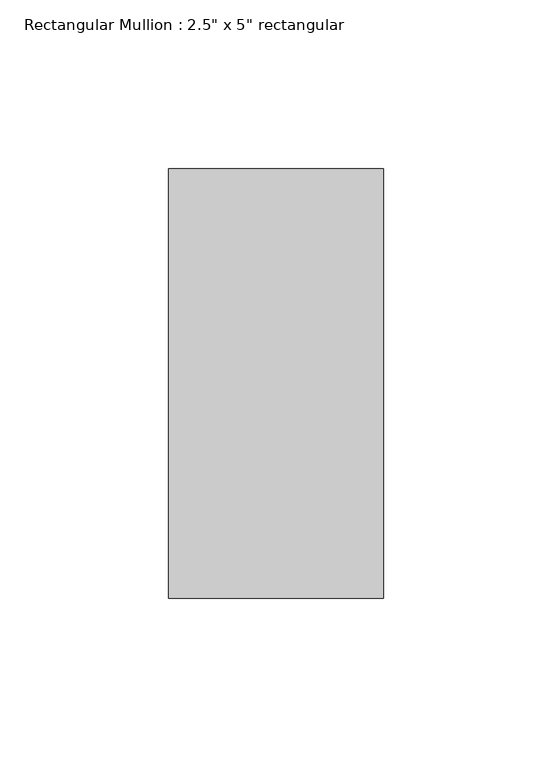
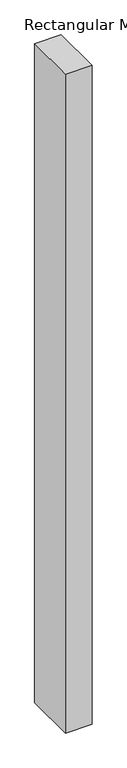
"""IFC4 building model written with IfcOpenShell, lengths in millimetres: member geometry."""

from ifc_helpers import new_model, si_unit, frame, origin, place, context, project, spatial, polyline, outline, extrude, source, transform, mapped, element, save


def member_70ee0c71(model_context):
    return source(origin(), model_context, "Body", "SweptSolid", [
        extrude(outline(polyline([(0.0, 63.5), (0.0, -63.5), (-63.5, -63.5), (-63.5, 63.5), (0.0, 63.5)])), frame((0.0, 0.0, -1665.3902237), z_axis=(0.0, 0.0, 1.0), x_axis=(1.0, 0.0, 0.0)), (0.0, 0.0, 1.0), 1665.3902237),
    ])


if __name__ == "__main__":
    model = new_model("IFC4")
    model_context = context("Model", 3, world=origin())
    ifc_project = project(units=[si_unit("LENGTHUNIT", "METRE", prefix="MILLI")], contexts=[model_context])
    site = spatial("IfcSite", under=ifc_project)
    building = spatial("IfcBuilding", under=site)
    placement = place(None, origin())
    member_shape = member_70ee0c71(model_context)
    element("IfcMember", 1, ObjectType="Rectangular Mullion : 2.5\" x 5\" rectangular", at=placement, inside=building, context=model_context, shape_type="MappedRepresentation", body=[
        mapped(member_shape, transform((0.0, 0.0, 0.0), x_axis=(1.0, 0.0, 0.0), y_axis=(0.0, 1.0, 0.0), z_axis=(0.0, 0.0, 1.0))),
    ])
    save(model, "model.ifc")

# Revit data of these elements
# Type "Rectangular Mullion : 2.5\" x 5\" rectangular"
#   built-in parameter 1007304 = 0.416667 (stored number, unit not read)
#   built-in parameter 1007301 = 0.104167 (stored number, unit not read)
#   built-in parameter 1007300 = 0.104167 (stored number, unit not read)
# Element 1 (IfcMember, "Rectangular Mullion : 2.5\" x 5\" rectangular")
#   Materials on its faces: "Aluminum"
# Materials
#   "Aluminum": class "Metal", colour RGB 247 247 247, transparency 0, Description = "Aluminum 6061", Cost = 0
